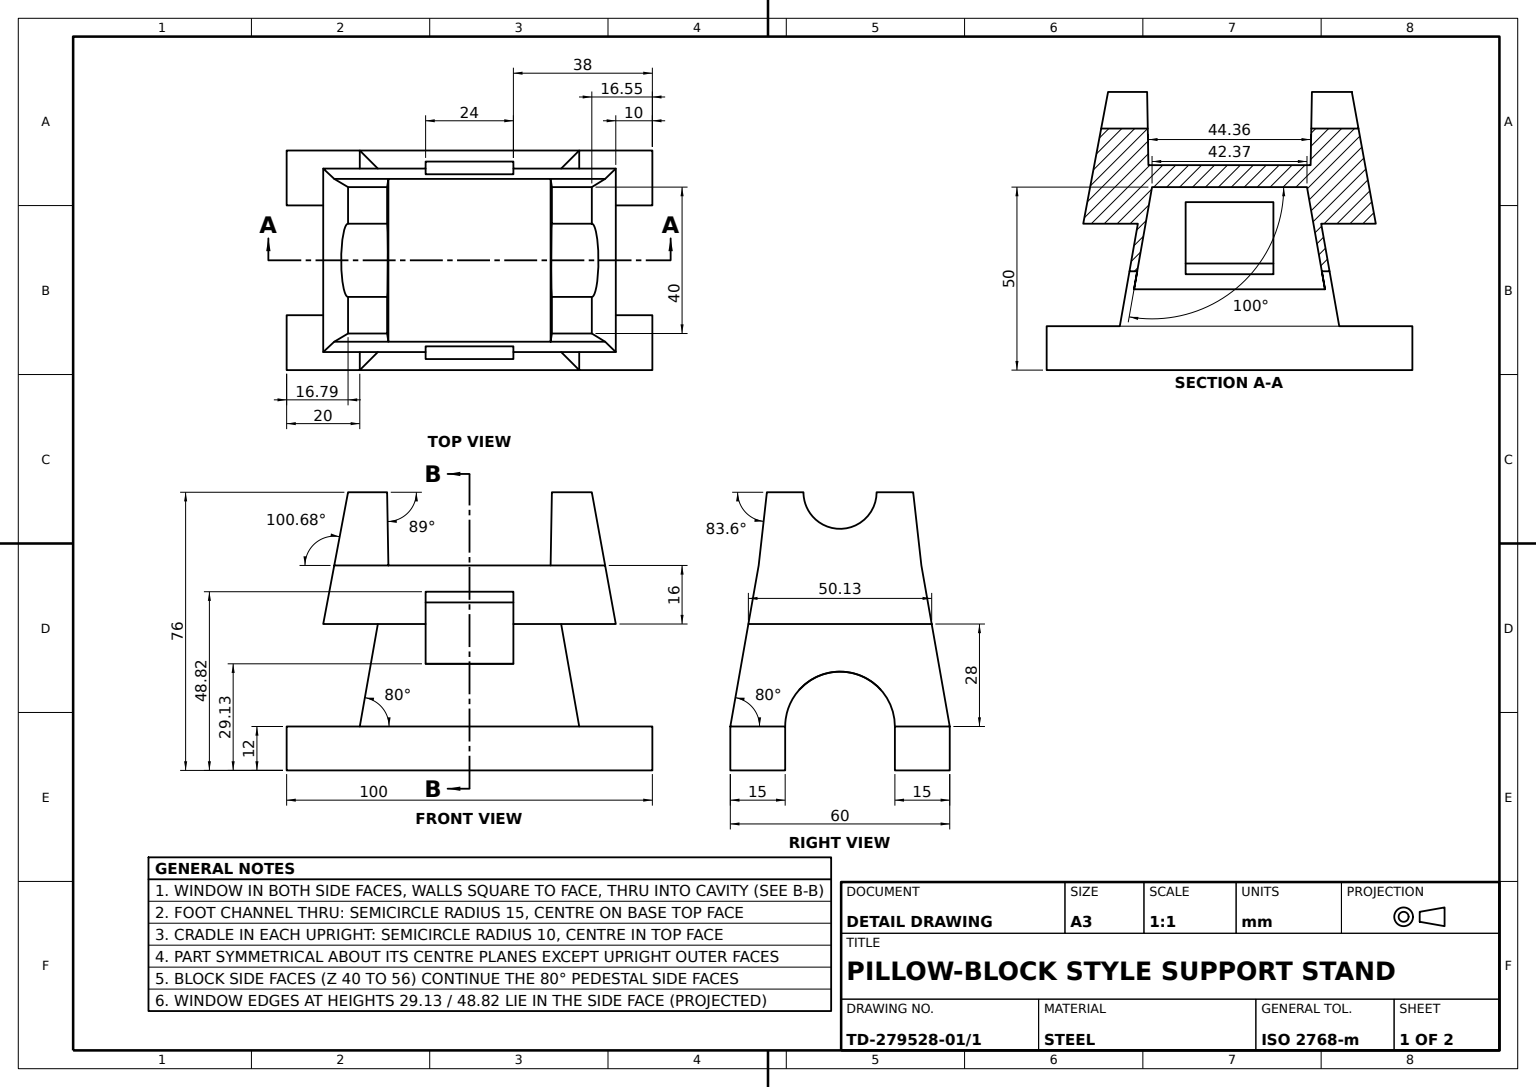
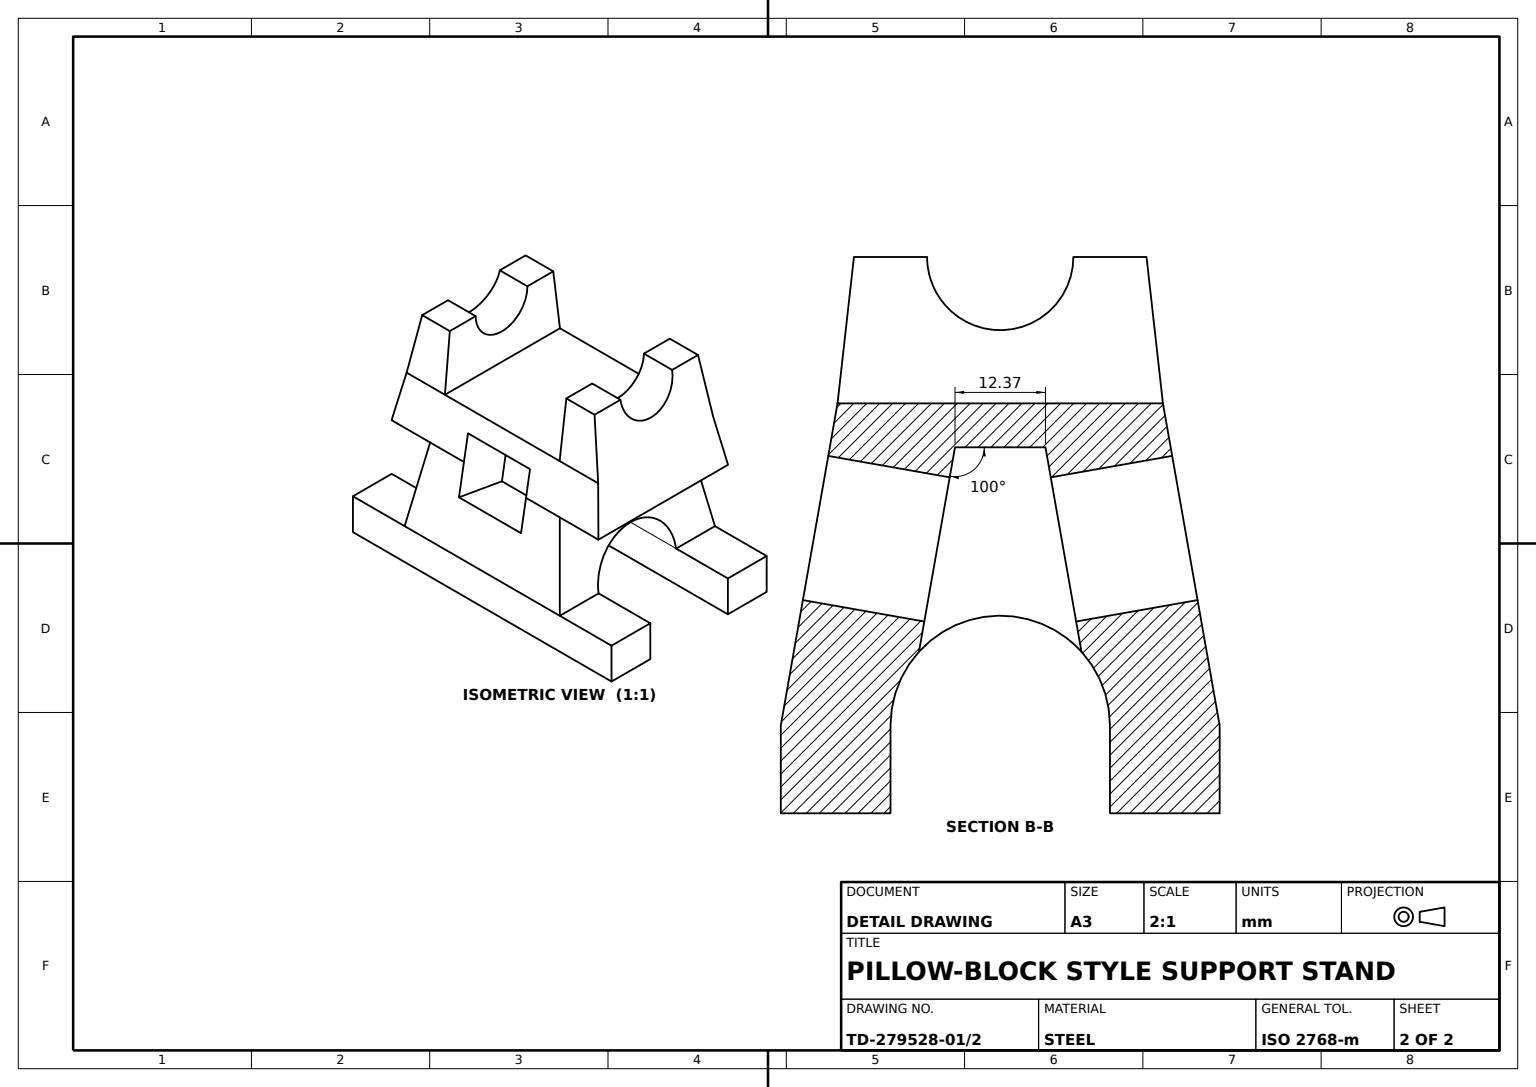
from build123d import *

# Parameters (mm, degrees)
BASE_PLATE_SKETCH_W            = 60
BASE_PLATE_SKETCH_H            = 100
BASE_PLATE_100X60X12_DEPTH     = 12
PEDESTAL_SKETCH_W              = 60
PEDESTAL_SKETCH_H              = 60
TAPERED_PEDESTAL_DEPTH         = 28
TAPERED_PEDESTAL_TAPER         = 10
FOOT_CHANNEL_SKETCH_W          = 30
FOOT_CHANNEL_SKETCH_H          = 12
FOOT_CHANNEL_CUT_DEPTH         = 200
UPPER_BLOCK_SKETCH_W           = 50.13
UPPER_BLOCK_SKETCH_H           = 80
UPPER_BLOCK_80X50_DEPTH        = 16
UPPER_BLOCK_80X50_TAPER        = 10
TOP_SLOT_SKETCH_W              = 24
TOP_SLOT_SKETCH_H              = 8.960181453
TOP_SLOT_CUT_DEPTH             = 16
PEDESTAL_RELIEF_SKETCH_W       = 30
PEDESTAL_RELIEF_SKETCH_H       = 60
PEDESTAL_RELIEF_CUT_DEPTH      = 50
PEDESTAL_RELIEF_CUT_DRAFT      = -10
WINDOW_SKETCH_W                = 24
WINDOW_SKETCH_H                = 20
SQUARE_WINDOW_20X20_DEPTH      = 5
SIDE_POCKET_SKETCH_W           = 24
SIDE_POCKET_SKETCH_H           = 8.960181453
SIDE_POCKET_SKETCH_H_2         = 11.039818547
SIDE_POCKET_CUT_DEPTH          = 20
RIB_BOSS_SKETCH_W              = 44.487536618
RIB_BOSS_SKETCH_H              = 74.357536618
RIB_BOSS_DEPTH                 = 20
RIB_BOSS_TAPER                 = 10
TRIM_CUT_DEPTH                 = 100
UPRIGHTS_SKETCH_W              = 44.487536618
UPRIGHTS_SKETCH_H              = 15
UPRIGHTS_15X15_DEPTH           = 20
UPRIGHTS_15X15_DRAFT           = 1
UPRIGHTS_15X15_PROFILE_2_DEPTH = 20
UPRIGHTS_15X15_PROFILE_2_DRAFT = 1
CRADLE_CUT_A_DEPTH             = 200
CRADLE_CUT_B_DEPTH             = 200
CROSS_BORE_CUT_DEPTH           = 100


with BuildPart() as part:
    # Base Plate Sketch → Base Plate 100x60x12 (new body)
    with BuildSketch(Plane(origin=(0, 0, 0), x_dir=(1, 0, 0), z_dir=(0, 1, 0))):
        Rectangle(BASE_PLATE_SKETCH_W, BASE_PLATE_SKETCH_H)
    extrude(amount=BASE_PLATE_100X60X12_DEPTH)

    # Pedestal Sketch → Tapered Pedestal (add)
    with BuildSketch(Plane(origin=(0, 12, 0), x_dir=(1, 0, 0), z_dir=(0, 1, 0))):
        Rectangle(PEDESTAL_SKETCH_W, PEDESTAL_SKETCH_H)
    extrude(amount=TAPERED_PEDESTAL_DEPTH, taper=TAPERED_PEDESTAL_TAPER)

    # Foot Channel Sketch → Foot Channel Cut (cut)
    with BuildSketch(Plane.XY.offset(50)):
        with BuildLine():
            ThreePointArc((15, 12), (0, 27), (-15, 12))
            Line((-15, 12), (15, 12))
        make_face()
        with Locations((0, 6)):
            Rectangle(FOOT_CHANNEL_SKETCH_W, FOOT_CHANNEL_SKETCH_H)
    extrude(amount=-FOOT_CHANNEL_CUT_DEPTH, mode=Mode.SUBTRACT)

    # Upper Block Sketch → Upper Block 80x50 (add)
    with BuildSketch(Plane(origin=(0, 40, 0), x_dir=(1, 0, 0), z_dir=(0, 1, 0))):
        Rectangle(UPPER_BLOCK_SKETCH_W, UPPER_BLOCK_SKETCH_H)
    extrude(amount=UPPER_BLOCK_80X50_DEPTH, taper=UPPER_BLOCK_80X50_TAPER)

    # Top Slot Sketch → Top Slot Cut (cut)
    with BuildSketch(Plane(origin=(31.149600637, 5.492515031, 0), x_dir=(0, 0, -1), z_dir=(0.9848077530122081, 0.17364817766693072, 0))):
        with Locations((0, 39.519909274)):
            Rectangle(TOP_SLOT_SKETCH_W, TOP_SLOT_SKETCH_H)
        Polygon((-12, 35.039818547), (-12, 24), (0, 24), (12, 24), (12, 35.039818547), align=None)
    extrude(amount=-TOP_SLOT_CUT_DEPTH, mode=Mode.SUBTRACT)


with BuildPart() as pedestal_relief_cut_tool:
    # Pedestal Relief Sketch → Pedestal Relief Cut (with draft: the straight prism first)
    with BuildSketch(Plane.XZ):
        Rectangle(PEDESTAL_RELIEF_SKETCH_W, PEDESTAL_RELIEF_SKETCH_H)
    extrude(amount=-PEDESTAL_RELIEF_CUT_DEPTH)
    # Pedestal Relief Cut: the draft: its side faces are tilted about the plane it starts from
    pedestal_relief_cut_sides = [pedestal_relief_cut_tool.faces().sort_by_distance(p)[0] for p in [
        (-15, 25, 0),
        (0, 25, -30),
        (15, 25, 0),
        (0, 25, 30),
    ]]
    draft(pedestal_relief_cut_sides, Plane.XZ, PEDESTAL_RELIEF_CUT_DRAFT)


with BuildPart() as part_1:
    add(part.part)

    # Pedestal Relief Cut: cut by pedestal_relief_cut_tool
    add(pedestal_relief_cut_tool.part, mode=Mode.SUBTRACT)

    # Window Sketch → Square Window 20x20 (cut)
    with BuildSketch(Plane(origin=(15.392676588, 2.714144188, 0), x_dir=(0, 0, -1), z_dir=(0.9848077530122081, 0.1736481776669307, 0))):
        with Locations((0, 34)):
            Rectangle(WINDOW_SKETCH_W, WINDOW_SKETCH_H)
    extrude(amount=-SQUARE_WINDOW_20X20_DEPTH, mode=Mode.SUBTRACT)

    # Side Pocket Sketch → Side Pocket Cut (cut)
    with BuildSketch(Plane(origin=(-31.149600637, 5.492515031, 0), x_dir=(0, 0, 1), z_dir=(-0.9848077530122081, 0.17364817766693072, 0))):
        with Locations((0, 39.519909274)):
            Rectangle(SIDE_POCKET_SKETCH_W, SIDE_POCKET_SKETCH_H)
        with Locations((0, 29.519909274)):
            Rectangle(SIDE_POCKET_SKETCH_W, SIDE_POCKET_SKETCH_H_2)
    extrude(amount=-SIDE_POCKET_CUT_DEPTH, mode=Mode.SUBTRACT)

    # Rib Boss Sketch → Rib Boss (add)
    with BuildSketch(Plane(origin=(0, 56, 0), x_dir=(1, 0, 0), z_dir=(0, 1, 0))):
        Rectangle(RIB_BOSS_SKETCH_W, RIB_BOSS_SKETCH_H)
    extrude(amount=RIB_BOSS_DEPTH, taper=RIB_BOSS_TAPER)

    # Trim Sketch → Trim Cut (cut)
    with BuildSketch(Plane.XY.offset(50)):
        Polygon((0, 56), (24.962521637, 56), (24.962521637, 76), (-29.161824343, 76), (-29.161824343, 56), align=None)
    extrude(amount=-TRIM_CUT_DEPTH, mode=Mode.SUBTRACT)


with BuildPart() as uprights_15x15_tool:
    # Uprights Sketch → Uprights 15x15 (with draft: the straight prism first)
    with BuildSketch(Plane(origin=(0, 56, 0), x_dir=(1, 0, 0), z_dir=(0, 1, 0))):
        with Locations((0, 29.678768309)):
            Rectangle(UPRIGHTS_SKETCH_W, UPRIGHTS_SKETCH_H)
    extrude(amount=UPRIGHTS_15X15_DEPTH)
    # Uprights 15x15: the draft: its side faces are tilted about the plane it starts from
    uprights_15x15_sides = [uprights_15x15_tool.faces().sort_by_distance(p)[0] for p in [
        (-22.243768309, 66, -29.678768309),
        (0, 66, -22.178768309),
        (22.243768309, 66, -29.678768309),
        (0, 66, -37.178768309),
    ]]
    draft(uprights_15x15_sides, Plane(origin=(0, 56, 0), x_dir=(1, 0, 0), z_dir=(0, 1, 0)), UPRIGHTS_15X15_DRAFT)


with BuildPart() as part_2:
    add(part_1.part)

    # Uprights 15x15: add uprights_15x15_tool
    add(uprights_15x15_tool.part)


with BuildPart() as uprights_15x15_profile_2_tool:
    # Uprights Sketch → Uprights 15x15 profile 2 (with draft: the straight prism first)
    with BuildSketch(Plane(origin=(0, 56, 0), x_dir=(1, 0, 0), z_dir=(0, 1, 0))):
        with Locations((0, -29.678768309)):
            Rectangle(UPRIGHTS_SKETCH_W, UPRIGHTS_SKETCH_H)
    extrude(amount=UPRIGHTS_15X15_PROFILE_2_DEPTH)
    # Uprights 15x15 profile 2: the draft: its side faces are tilted about the plane it starts from
    uprights_15x15_profile_2_sides = [uprights_15x15_profile_2_tool.faces().sort_by_distance(p)[0] for p in [
        (0, 66, 37.178768309),
        (22.243768309, 66, 29.678768309),
        (0, 66, 22.178768309),
        (-22.243768309, 66, 29.678768309),
    ]]
    draft(uprights_15x15_profile_2_sides, Plane(origin=(0, 56, 0), x_dir=(1, 0, 0), z_dir=(0, 1, 0)), UPRIGHTS_15X15_PROFILE_2_DRAFT)


with BuildPart() as part_3:
    add(part_2.part)

    # Uprights 15x15 profile 2: add uprights_15x15_profile_2_tool
    add(uprights_15x15_profile_2_tool.part)

    # Cradle Cut A Sketch → Cradle Cut A (cut)
    with BuildSketch(Plane.XY.offset(50)):
        Polygon((20, 76), (22.243768309, 56), (21.89466701, 76), align=None)
        Polygon((-22.243768309, 56), (-20, 76), (-21.89466701, 76), align=None)
    extrude(amount=-CRADLE_CUT_A_DEPTH, mode=Mode.SUBTRACT)

    # Cradle Cut B Sketch → Cradle Cut B (cut)
    with BuildSketch(Plane(origin=(30, 0, 0), x_dir=(0, 0, -1), z_dir=(1, 0, 0))):
        Polygon((-40, 40), (-33.208201883, 76), (-36.82966701, 76), align=None)
        Polygon((40, 40), (33.445403325, 76), (36.82966701, 76), align=None)
    extrude(amount=-CRADLE_CUT_B_DEPTH, mode=Mode.SUBTRACT)

    # Cross Bore Sketch → Cross Bore Cut (cut)
    with BuildSketch(Plane.XY.offset(50)):
        with BuildLine():
            Line((-10, 76), (10, 76))
            ThreePointArc((10, 76), (0, 66), (-10, 76))
        make_face()
    extrude(amount=-CROSS_BORE_CUT_DEPTH, mode=Mode.SUBTRACT)


solid = part_3.part
